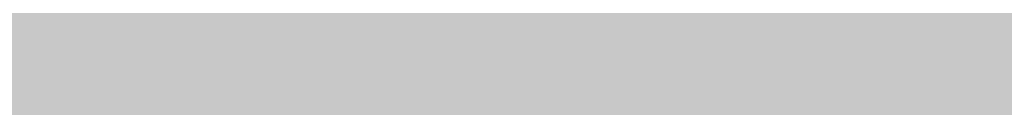
# Model space of a CAD drawing. Units: inches. Extents: x 2091 to 2899, y 967 to 2217.
# Tile 217 of 256: x 2203.2571 to 2203.4104, y 1152.2605 to 1152.274. Entities that reach past the tile are written whole.
import ezdxf

# ---------------------------------------------------------------- set-up
doc = ezdxf.new("R2010")
doc.units = ezdxf.units.IN
doc.layers.add('A-WALL-PATT', color=141, linetype='Continuous', lineweight=13, true_color=0xadddf7)

msp = doc.modelspace()

# ---------------------------------------------------------------- hatches: boundary and pattern name
at = {"layer": 'A-WALL-PATT'}
h = msp.add_hatch(color=256, dxfattribs=at)
h.dxf.hatch_style = 1
h.paths.add_polyline_path([(2803.1436, 2050.91906), (2203.1436, 2050.91906), (2203.1436, 1090.91906), (2803.1436, 1090.91906)])
h.paths.add_polyline_path([(2635.79885, 1147.54046), (2674.52405, 1147.54046, 0.376086), (2678.52967, 1152.8802), (2678.52967, 1159.55647, 0.333335), (2674.52432, 1163.56185), (2674.52432, 1163.56185), (2674.52432, 1192.93439), (2635.80597, 1192.93439), (2597.08762, 1192.93439), (2597.08762, 1163.56185, 0.333335), (2593.08228, 1159.55647), (2593.08228, 1152.8802, 0.376086), (2597.08789, 1147.54046)], flags=0)
h.paths.add_polyline_path([(2436.01043, 1278.24078, 0.000483), (2435.95264, 1278.21503, -0.001328), (2435.93563, 1278.11169, -0.001711), (2436.11644, 1278.04076, 0.002185)], flags=0)
h.paths.add_polyline_path([(2794.1436, 1143.41906), (2794.1436, 1347.41906), (2543.37017, 1347.41906), (2543.37017, 1351.91906), (2794.1436, 1351.91906), (2794.1436, 1392.71355), (2793.9474, 1392.71355), (2793.9474, 1473.5369), (2794.1436, 1473.5369), (2794.1436, 1531.91906), (2650.1436, 1531.91906), (2650.1436, 1536.41906), (2794.1436, 1536.41906), (2794.1436, 1692.41906), (2609.37561, 1692.41906), (2609.37561, 1644.41906), (2604.87561, 1644.41906), (2604.87561, 1744.91906), (2609.37561, 1744.91906), (2609.37561, 1696.91906), (2794.1436, 1696.91906), (2794.1436, 1780.91906), (2609.6436, 1780.91906), (2493.87561, 1780.91906), (2493.87561, 1785.41906), (2609.6436, 1785.41906), (2794.1436, 1785.41906), (2794.1436, 1847.93882), (2793.95122, 1847.93882), (2793.95122, 1928.76217), (2794.1436, 1928.76217), (2794.1436, 1941.41906), (2614.1436, 1941.41906), (2614.1436, 1821.41906), (2609.6436, 1821.41906), (2609.6436, 1941.41906), (2392.1436, 1941.41906), (2392.1436, 1819.91906), (2387.6436, 1819.91906), (2387.6436, 1941.41906), (2212.1436, 1941.41906), (2212.1436, 1783.91906), (2392.1436, 1783.91906), (2392.1436, 1780.91906), (2212.1436, 1780.91906), (2212.1436, 1629.41906), (2387.6436, 1629.41906), (2387.6436, 1744.91906), (2392.1436, 1744.91906), (2392.1436, 1627.91906), (2317.1436, 1627.91906), (2317.1436, 1551.41906), (2317.1436, 1536.41906), (2459.38359, 1536.41906), (2459.38359, 1602.39648), (2463.88359, 1602.39648), (2463.88359, 1531.91906), (2456.6436, 1531.91906), (2456.6436, 1529.91906), (2452.1436, 1529.91906), (2452.1436, 1531.91906), (2312.6436, 1531.91906), (2312.6436, 1551.41906), (2306.1436, 1551.41906), (2306.1436, 1555.91906), (2308.1436, 1555.91906), (2308.1436, 1551.41906), (2312.6436, 1551.41906), (2312.6436, 1627.91906), (2212.1436, 1627.91906), (2212.1436, 1555.91906), (2270.1436, 1555.91906), (2270.1436, 1551.41906), (2212.1436, 1551.41906), (2212.1436, 1351.91906), (2272.1436, 1351.91906), (2272.1436, 1347.41906), (2212.1436, 1347.41906), (2212.1436, 1275.41906), (2308.1436, 1275.41906), (2308.1436, 1351.91906), (2452.1436, 1351.91906), (2452.1436, 1493.91906), (2456.6436, 1493.91906), (2456.6436, 1347.41906), (2312.6436, 1347.41906), (2312.6436, 1270.91906), (2212.1436, 1270.91906), (2212.1436, 1099.91906), (2281.23752, 1099.91906), (2282.87104, 1110.9138), (2282.00834, 1116.9966), (2278.55774, 1121.4204), (2268.20564, 1128.0562), (2272.08764, 1128.0562), (2273.81294, 1131.927), (2279.42034, 1134.6919), (2285.02784, 1135.2449), (2287.61584, 1137.4568), (2288.04714, 1138.0098), (2289.34114, 1140.7747), (2291.06654, 1139.6687), (2292.36054, 1135.2449), (2295.37984, 1136.9038), (2296.24254, 1135.7979), (2297.10524, 1133.033), (2300.12464, 1138.0098), (2303.14394, 1138.0098), (2304.43794, 1135.7979), (2303.14394, 1133.586), (2306.59464, 1134.6919), (2307.88874, 1133.033), (2310.90804, 1135.2449), (2313.92744, 1134.1389), (2315.62686, 1132.4271), (2308.32004, 1117.5496), (2290.20384, 1109.8079), (2288.90984, 1103.1721), (2289.27231, 1099.91906), (2434.91823, 1099.91906), (2431.59323, 1124.78806), (2429.93023, 1169.55306), (2430.92718, 1240.51969), (2435.65893, 1238.18613), (2437.13523, 1196.55406), (2438.79823, 1143.97306), (2442.67823, 1111.99806), (2446.55823, 1099.91906), (2794.1436, 1099.91906), (2794.1436, 1138.91906), (2548.03245, 1138.91906), (2548.03245, 1143.41906), (2548.03245, 1148.81906), (2546.66846, 1148.03156), (2528.68569, 1179.17862, 0.256256), (2512.03245, 1148.81906), (2512.03245, 1143.41906), (2512.03245, 1138.91906), (2507.53245, 1138.91906), (2507.53245, 1143.41906), (2507.53245, 1148.81906, 0.256256), (2490.8792, 1179.17862), (2472.89644, 1148.03156), (2471.53245, 1148.81906), (2471.53245, 1143.41906), (2467.03245, 1143.41906), (2467.03245, 1269.94579, 0.039061), (2460.90999, 1273.58006), (2467.03245, 1273.58006), (2467.03245, 1286.32536, 0.014511), (2465.21619, 1286.76191), (2467.03245, 1287.05258), (2467.03245, 1323.41906), (2471.53245, 1323.41906), (2471.53245, 1148.81906), (2489.53245, 1179.99597), (2490.89644, 1179.20847), (2490.8792, 1179.17862, -0.256256), (2507.53245, 1148.81906), (2507.53245, 1143.41906), (2512.03245, 1143.41906), (2512.03245, 1148.81906, -0.256256), (2528.68569, 1179.17862), (2528.66846, 1179.20847), (2530.03245, 1179.99597), (2548.03245, 1148.81906), (2548.03245, 1143.41906)], flags=16)
h.paths.add_polyline_path([(2607.76855, 1200.94508), (2607.76855, 1265.03063), (2597.08762, 1281.05201), (2619.78459, 1281.05201), (2627.79528, 1337.12686), (2635.79885, 1337.12686), (2643.81666, 1337.12686), (2651.82736, 1281.05201), (2674.52432, 1281.05201), (2663.8434, 1265.03063), (2663.8434, 1200.94508), (2635.80597, 1200.94508)], flags=0)
edge = h.paths.add_edge_path(flags=0)
edge.add_ellipse((13303.89622, 1272.99872), major_axis=(-10595.31304, 0), ratio=0.84230387009, start_angle=0.628237219, end_angle=0.6465541, ccw=False)
edge.add_ellipse((2711.70045, 1156.85268), major_axis=(2.21977, 0), ratio=0.8423039, start_angle=111.53524, end_angle=180.62824, ccw=False)
edge.add_ellipse((13303.15629, 1272.99872), major_axis=(-10593.02631, 0), ratio=0.84230386954, start_angle=0.528271472, end_angle=0.646554097, ccw=False)
edge.add_line((2710.7646, 1175.3333), (2710.12999, 1175.3333))
edge.add_ellipse((2710.12999, 1176.57978), major_axis=(1.47985, 0), ratio=0.8423039, start_angle=180, end_angle=270, ccw=False)
edge.add_line((2708.65014, 1176.57978), (2708.65014, 1200.78291))
edge.add_ellipse((2710.12999, 1200.78291), major_axis=(1.47985, 0), ratio=0.8423039, start_angle=90, end_angle=180, ccw=False)
edge.add_line((2710.12999, 1202.02939), (2710.46508, 1202.02939))
edge.add_ellipse((13303.15629, 1272.99872), major_axis=(-10593.02631, 0), ratio=0.84230386954, start_angle=-0.090229089, end_angle=0.383866779, ccw=False)
edge.add_ellipse((2710.12999, 1290.92703), major_axis=(-1.47985, 0), ratio=0.8423039, start_angle=0, end_angle=90, ccw=False)
edge.add_line((2708.65014, 1290.92703), (2708.65014, 1315.13017))
edge.add_ellipse((2710.12999, 1315.13017), major_axis=(-1.47985, 0), ratio=0.8423039, start_angle=-90, end_angle=0, ccw=False)
edge.add_line((2710.12999, 1316.37665), (2710.70631, 1316.37665))
edge.add_ellipse((3238.40172, 1296.28957), major_axis=(528.234, 0), ratio=0.84230387, start_angle=176.3495724, end_angle=177.8200497, ccw=False)
edge.add_ellipse((2775.06304, 1071.4507), major_axis=(313.30776, 0), ratio=0.84230387, start_angle=102.1259656, end_angle=103.780529, ccw=False)
edge.add_ellipse((2775.06304, 1078.3057), major_axis=(-305.30289, 0), ratio=0.84230387, start_angle=-79.790461, end_angle=-77.5553727, ccw=False)
edge.add_ellipse((2695.14177, 1541.97538), major_axis=(-250.96022, 0), ratio=0.84230387, start_angle=99.256566, end_angle=102.5549326)
edge.add_line((2741.41033, 1334.21426), (2747.13255, 1337.37848))
edge.add_ellipse((2747.53862, 1336.85748), major_axis=(-0.73992, 0), ratio=0.842304, start_angle=270, end_angle=307.93313, ccw=False)
edge.add_ellipse((2747.53862, 1336.85748), major_axis=(-0.73992, 0), ratio=0.842304, start_angle=232.06687, end_angle=270, ccw=False)
edge.add_line((2747.94469, 1337.37848), (2753.66691, 1334.21426))
edge.add_ellipse((2799.93547, 1541.97538), major_axis=(250.96022, 0), ratio=0.84230387, start_angle=257.4450674, end_angle=260.743434)
edge.add_ellipse((2720.01419, 1078.3057), major_axis=(305.30289, 0), ratio=0.84230387, start_angle=77.5553727, end_angle=79.790461, ccw=False)
edge.add_ellipse((2720.01419, 1071.4507), major_axis=(-313.30776, 0), ratio=0.84230387, start_angle=256.219471, end_angle=257.8740344, ccw=False)
edge.add_ellipse((2256.67551, 1296.28957), major_axis=(-528.234, 0), ratio=0.84230387, start_angle=182.1799503, end_angle=183.6504276, ccw=False)
edge.add_line((2784.37092, 1316.37665), (2784.94725, 1316.37665))
edge.add_ellipse((2784.94725, 1315.13017), major_axis=(1.47985, 0), ratio=0.8423039, start_angle=0, end_angle=90, ccw=False)
edge.add_line((2786.42709, 1315.13017), (2786.42709, 1290.92703))
edge.add_ellipse((2784.94725, 1290.92703), major_axis=(1.47985, 0), ratio=0.8423039, start_angle=270, end_angle=360, ccw=False)
edge.add_ellipse((-7808.07906, 1272.99872), major_axis=(10593.02631, 0), ratio=0.84230386954, start_angle=-0.383866779, end_angle=0.090229089, ccw=False)
edge.add_line((2784.61216, 1202.02939), (2784.94725, 1202.02939))
edge.add_ellipse((2784.94725, 1200.78291), major_axis=(1.47985, 0), ratio=0.8423039, start_angle=0, end_angle=90, ccw=False)
edge.add_line((2786.42709, 1200.78291), (2786.42709, 1176.57978))
edge.add_ellipse((2784.94725, 1176.57978), major_axis=(-1.47985, 0), ratio=0.8423039, start_angle=90, end_angle=180, ccw=False)
edge.add_line((2784.94725, 1175.3333), (2784.31264, 1175.3333))
edge.add_ellipse((-7808.07906, 1272.99872), major_axis=(10593.02631, 0), ratio=0.84230386954, start_angle=-0.618643196, end_angle=-0.528271472, ccw=False)
edge.add_ellipse((2783.37678, 1156.85268), major_axis=(-2.21977, 0), ratio=0.8423039, start_angle=179.37176, end_angle=248.46476, ccw=False)
edge.add_ellipse((-7808.81898, 1272.99872), major_axis=(-10595.31304, 0), ratio=0.84230386576, start_angle=179.353445923, end_angle=179.371762803, ccw=False)
edge.add_ellipse((2780.2973, 1153.50079), major_axis=(-5.24643, 0), ratio=0.8423039, start_angle=90, end_angle=179.35345, ccw=False)
edge.add_line((2780.2973, 1149.08171), (2714.77993, 1149.08171))
edge.add_ellipse((2714.77993, 1153.50079), major_axis=(5.24643, 0), ratio=0.8423039, start_angle=180.64655, end_angle=270, ccw=False)
edge = h.paths.add_edge_path(flags=0)
edge.add_line((2718.18737, 1151.00783), (2718.18737, 1170.47236))
edge.add_ellipse((2721.14706, 1170.47236), major_axis=(-2.95969, 0), ratio=0.8423039, start_angle=-90, end_angle=0, ccw=False)
edge.add_line((2721.14706, 1172.96532), (2773.93017, 1172.96532))
edge.add_ellipse((2773.93017, 1170.47236), major_axis=(-2.95969, 0), ratio=0.8423039, start_angle=180, end_angle=270, ccw=False)
edge.add_line((2776.88987, 1170.47236), (2776.88987, 1151.00783))
edge.add_line((2776.88987, 1151.00783), (2718.18737, 1151.00783))
edge = h.paths.add_edge_path(flags=0)
edge.add_line((2718.18737, 1180.23415), (2718.18737, 1199.05783))
edge.add_ellipse((2747.53862, 1320.39864), major_axis=(147.01792, 0), ratio=0.84230387, start_angle=256.4018653, end_angle=283.5981347)
edge.add_line((2776.88987, 1199.05783), (2776.88987, 1180.23415))
edge.add_ellipse((2747.53862, 1301.57496), major_axis=(147.01792, 0), ratio=0.84230387, start_angle=256.4018653, end_angle=283.5981347, ccw=False)
edge = h.paths.add_edge_path(flags=0)
edge.add_ellipse((13303.15629, 1272.99872), major_axis=(-10591.54646, 0), ratio=0.84230386955, start_angle=0.055594314, end_angle=0.377764194, ccw=False)
edge.add_line((2711.61686, 1262.72171), (2715.66741, 1249.4954))
edge.add_ellipse((6413.89196, 1241.69192), major_axis=(-3698.23616, 0), ratio=0.8423038695, start_angle=-0.12089737, end_angle=0.36407635)
edge.add_line((2715.76104, 1218.19245), (2711.93431, 1203.16736))
edge = h.paths.add_edge_path(flags=0)
edge.add_line((2718.18737, 1251.07457), (2716.00249, 1267.45044))
edge.add_ellipse((2742.15117, 1202.18954), major_axis=(81.77258, 0), ratio=0.84230387, start_angle=94.277421, end_angle=111.8349538, ccw=False)
edge.add_line((2737.00975, 1270.93063), (2758.06748, 1270.93063))
edge.add_ellipse((2752.92606, 1202.18954), major_axis=(81.77258, 0), ratio=0.84230387, start_angle=68.1650462, end_angle=85.722579, ccw=False)
edge.add_line((2779.07475, 1267.45044), (2776.88987, 1251.07457))
edge.add_ellipse((2750.33806, 1187.88536), major_axis=(79.57966, 0), ratio=0.84230387, start_angle=67.2080851, end_angle=85.1299304)
edge.add_line((2756.03466, 1254.74366), (2739.04258, 1254.74366))
edge.add_ellipse((2744.73917, 1187.88536), major_axis=(79.57966, 0), ratio=0.84230387, start_angle=94.8700696, end_angle=112.7919149)
edge = h.paths.add_edge_path(flags=0)
edge.add_line((2783.14293, 1203.16736), (2779.31619, 1218.19245))
edge.add_ellipse((-918.81473, 1241.69192), major_axis=(3698.23616, 0), ratio=0.8423038695, start_angle=-0.36407635, end_angle=0.12089737)
edge.add_line((2779.40983, 1249.4954), (2783.46037, 1262.72171))
edge.add_ellipse((-7808.07906, 1272.99872), major_axis=(-10591.54646, 0), ratio=0.84230386954, start_angle=179.622235806, end_angle=179.944405687, ccw=False)
edge = h.paths.add_edge_path(flags=0)
edge.add_ellipse((2734.20089, 1286.69044), major_axis=(-0.35661, 6.34008), ratio=0.6038336, start_angle=89.002014, end_angle=253.657408, ccw=False)
edge.add_line((2730.369, 1286.54181), (2730.369, 1301.35198))
edge.add_line((2730.369, 1301.35198), (2735.91331, 1305.2148))
edge.add_ellipse((2736.38492, 1304.73456), major_axis=(0.73992, 0), ratio=0.842304, start_angle=90, end_angle=134.48021, ccw=False)
edge.add_line((2736.38492, 1305.3578), (2738.03278, 1305.3578))
edge.add_line((2738.03278, 1305.3578), (2738.03278, 1307.70793))
edge.add_ellipse((2794.20164, 1307.70793), major_axis=(56.16886, 0), ratio=0.84230387, start_angle=150.56143, end_angle=180, ccw=False)
edge.add_ellipse((2700.87559, 1307.70793), major_axis=(-56.16886, 0), ratio=0.84230387, start_angle=180, end_angle=209.43857, ccw=False)
edge.add_line((2757.04445, 1307.70793), (2757.04445, 1305.3578))
edge.add_line((2757.04445, 1305.3578), (2758.69232, 1305.3578))
edge.add_ellipse((2758.69232, 1304.73456), major_axis=(-0.73992, 0), ratio=0.842304, start_angle=225.51979, end_angle=270, ccw=False)
edge.add_line((2759.16392, 1305.2148), (2764.70823, 1301.35198))
edge.add_line((2764.70823, 1301.35198), (2764.70823, 1286.54181))
edge.add_ellipse((2760.87634, 1286.69044), major_axis=(0.35661, 6.34008), ratio=0.6038336, start_angle=106.342592, end_angle=270.997986, ccw=False)
edge.add_line((2757.04445, 1285.79709), (2757.04445, 1307.70793))
edge.add_ellipse((2700.87559, 1307.70793), major_axis=(-56.16886, 0), ratio=0.84230387, start_angle=180, end_angle=209.43857)
edge.add_ellipse((2794.20164, 1307.70793), major_axis=(56.16886, 0), ratio=0.84230387, start_angle=150.56143, end_angle=180)
edge.add_line((2738.03278, 1307.70793), (2738.03278, 1285.79709))
h.paths.add_polyline_path([(2417.81227, 1104.4497), (2413.49227, 1102.5297), (2410.61227, 1103.9697), (2409.17227, 1106.3697), (2407.25227, 1107.3297), (2406.29227, 1109.7297), (2405.33227, 1114.0497), (2405.33227, 1117.8897), (2406.29227, 1120.1297), (2407.25227, 1119.8097), (2408.84832, 1118.32766), (2410.17395, 1119.42417), (2410.21127, 1120.4057), (2411.04073, 1121.41905), (2410.69927, 1119.8587), (2410.17395, 1119.42417), (2410.08845, 1117.17611), (2411.13284, 1116.20632), (2413.97227, 1119.3297), (2416.85227, 1120.7697), (2416.86972, 1120.79878), (2417.03507, 1119.40512), (2417.89621, 1118.14338), (2418.29227, 1118.3697), (2419.54445, 1120.03927), (2419.36092, 1118.38749), (2419.03211, 1119.35615), (2418.39894, 1118.51193), (2419.25227, 1114.5297), (2418.79409, 1107.19879)], flags=0)
h.paths.add_polyline_path([(2508.87017, 1347.41906), (2508.37017, 1347.41906), (2508.37017, 1351.91906), (2508.87017, 1351.91906)], flags=0)
h.paths.add_polyline_path([(2473.37017, 1347.41906), (2472.37017, 1347.41906), (2467.87017, 1347.41906), (2467.87017, 1455.41906), (2472.37017, 1455.41906), (2472.37017, 1352.41906), (2473.37017, 1352.41906)], flags=0)
h.paths.add_polyline_path([(2352.10624, 1217.4462), (2349.22624, 1218.8862), (2347.78624, 1221.2862), (2345.86624, 1222.2462), (2344.90624, 1224.6462), (2343.94624, 1228.9662), (2343.94624, 1232.8062), (2344.90624, 1235.0462), (2345.86624, 1234.7262), (2347.46229, 1233.24415), (2348.78792, 1234.34066), (2348.82524, 1235.3222), (2349.6547, 1236.33555), (2349.31324, 1234.7752), (2348.78792, 1234.34066), (2348.70242, 1232.0926), (2349.74681, 1231.12282), (2352.58624, 1234.2462), (2355.46624, 1235.6862), (2355.48369, 1235.71528), (2355.64904, 1234.32161), (2356.51018, 1233.05988), (2356.90624, 1233.2862), (2358.15842, 1234.95576), (2357.97489, 1233.30398), (2357.64608, 1234.27264), (2357.01291, 1233.42842), (2357.86624, 1229.4462), (2357.40806, 1222.11529), (2356.42624, 1219.3662)], flags=0)
h.paths.add_polyline_path([(2348.2968, 1112.22442), (2347.0138, 1112.31042), (2345.5298, 1114.12742), (2345.7318, 1115.85842), (2346.8118, 1116.98242), (2346.8118, 1114.64642), (2345.8668, 1114.21442), (2346.8798, 1114.30042)], flags=0)
h.paths.add_polyline_path([(2347.0138, 1110.92642), (2346.2718, 1110.49342), (2346.6098, 1111.18642)], flags=0)
h.paths.add_polyline_path([(2345.8668, 1118.19442), (2345.5298, 1117.32942), (2343.7078, 1118.02142), (2344.3828, 1118.62642)], flags=0)
h.paths.add_polyline_path([(2346.6768, 1109.28242), (2346.0698, 1108.07142), (2345.8668, 1110.06142)], flags=0)
h.paths.add_polyline_path([(2345.0568, 1119.75142), (2343.6398, 1119.75142), (2343.9778, 1121.13542)], flags=0)
h.paths.add_polyline_path([(2345.2598, 1116.55042), (2345.1248, 1115.85842), (2344.9218, 1115.68542), (2344.7198, 1116.37742)], flags=0)
h.paths.add_polyline_path([(2345.6648, 1112.31042), (2345.4618, 1111.53242), (2344.0448, 1111.96442), (2344.6518, 1112.57042)], flags=0)
h.paths.add_polyline_path([(2345.1918, 1113.34942), (2344.4498, 1113.86842), (2344.7198, 1114.38742)], flags=0)
h.paths.add_polyline_path([(2344.6518, 1116.80942), (2344.1798, 1115.68542), (2344.6518, 1115.33942), (2343.9098, 1114.90642), (2343.0328, 1115.94442), (2343.6398, 1116.46342)], flags=0)
h.paths.add_polyline_path([(2345.8668, 1106.68642), (2344.9898, 1105.56242), (2344.5168, 1106.60042)], flags=0)
h.paths.add_polyline_path([(2344.8548, 1110.06142), (2344.5168, 1109.28242), (2344.1128, 1109.71542)], flags=0)
h.paths.add_polyline_path([(2344.0448, 1113.52242), (2343.4378, 1113.08942), (2342.7628, 1113.95442)], flags=0)
h.paths.add_polyline_path([(2344.3148, 1111.01242), (2342.9648, 1110.32042), (2342.9648, 1111.09942)], flags=0)
h.paths.add_polyline_path([(2345.1248, 1104.69742), (2344.5848, 1103.74542), (2344.4498, 1104.26442)], flags=0)
h.paths.add_polyline_path([(2342.8298, 1121.22242), (2341.7498, 1120.53042), (2340.5358, 1121.04942), (2340.1308, 1121.82842), (2340.6708, 1122.95242), (2341.1428, 1121.82842), (2341.6148, 1122.00142)], flags=0)
h.paths.add_polyline_path([(2342.9648, 1119.75142), (2343.0328, 1118.45342), (2342.0878, 1118.02142), (2342.0198, 1119.49142)], flags=0)
h.paths.add_polyline_path([(2342.6948, 1116.89642), (2341.9528, 1116.63642), (2342.0198, 1117.32942)], flags=0)
h.paths.add_polyline_path([(2343.0328, 1112.22442), (2342.0198, 1111.79142), (2341.5478, 1112.22442), (2342.3578, 1113.34942)], flags=0)
h.paths.add_polyline_path([(2343.7748, 1104.43742), (2342.6278, 1102.88042), (2342.6948, 1104.61042), (2343.4378, 1105.12942)], flags=0)
h.paths.add_polyline_path([(2342.0198, 1115.07942), (2340.8058, 1115.51242), (2340.9408, 1116.37742)], flags=0)
h.paths.add_polyline_path([(2341.4808, 1120.09742), (2341.4808, 1119.40542), (2341.0758, 1119.57842), (2341.1428, 1120.09742)], flags=0)
h.paths.add_polyline_path([(2341.8178, 1114.47342), (2340.9408, 1113.08942), (2340.8058, 1114.56042)], flags=0)
h.paths.add_polyline_path([(2341.1428, 1118.54042), (2340.9408, 1116.98242), (2339.0508, 1117.67542), (2339.0508, 1118.62642)], flags=0)
h.paths.add_polyline_path([(2342.6948, 1101.66842), (2341.9528, 1101.84142), (2342.5598, 1102.36142)], flags=0)
h.paths.add_polyline_path([(2340.3328, 1119.66542), (2338.4438, 1119.57842), (2337.9038, 1120.35742), (2339.6578, 1120.61642)], flags=0)
h.paths.add_polyline_path([(2340.3328, 1115.33942), (2340.0628, 1113.69542), (2339.3878, 1115.33942)], flags=0)
h.paths.add_polyline_path([(2341.8178, 1103.83142), (2341.5478, 1102.88042), (2341.1428, 1103.65842)], flags=0)
h.paths.add_polyline_path([(2339.0508, 1122.86642), (2337.2958, 1121.82842), (2337.0938, 1123.12542), (2337.7688, 1123.81842)], flags=0)
h.paths.add_polyline_path([(2339.1178, 1121.74142), (2338.8478, 1121.22242), (2338.1738, 1121.04942), (2338.3758, 1121.56842)], flags=0)
h.paths.add_polyline_path([(2339.1858, 1119.31942), (2338.6458, 1118.71342), (2338.2408, 1118.10742), (2338.2408, 1118.88642)], flags=0)
h.paths.add_polyline_path([(2341.1428, 1101.92842), (2340.6028, 1101.23642), (2340.0628, 1101.84142), (2340.6028, 1102.36142)], flags=0)
h.paths.add_polyline_path([(2337.6338, 1117.76142), (2336.6208, 1118.28042), (2337.2958, 1118.97242)], flags=0)
h.paths.add_polyline_path([(2336.8238, 1119.57842), (2334.7988, 1118.97242), (2335.2038, 1120.35742), (2336.5538, 1120.87642)], flags=0)
h.paths.add_polyline_path([(2339.1178, 1100.45742), (2337.3638, 1100.54342), (2336.7558, 1101.23642)], flags=0)
h.paths.add_polyline_path([(2336.3508, 1122.43342), (2336.0138, 1121.91442), (2334.9338, 1122.43342), (2334.5288, 1123.47142), (2335.7438, 1122.77942)], flags=0)
h.paths.add_polyline_path([(2334.7318, 1120.87642), (2334.2588, 1120.35742), (2334.0568, 1120.78942), (2334.5968, 1121.30842)], flags=0)
h.paths.add_polyline_path([(2334.4618, 1122.17442), (2332.5718, 1121.30842), (2331.3568, 1122.17442), (2332.0998, 1122.86642)], flags=0)
h.paths.add_polyline_path([(2334.2588, 1118.54042), (2333.3818, 1118.45342), (2333.6518, 1119.31942)], flags=0)
h.paths.add_polyline_path([(2335.5418, 1102.27442), (2334.1918, 1102.62042), (2335.2718, 1103.31242)], flags=0)
h.paths.add_polyline_path([(2332.7068, 1119.66542), (2331.6948, 1120.44342), (2332.5048, 1120.78942)], flags=0)
h.paths.add_polyline_path([(2334.7318, 1101.14942), (2333.5168, 1101.58242), (2333.9888, 1101.75542)], flags=0)
h.paths.add_polyline_path([(2332.6398, 1116.63642), (2331.0868, 1116.29042), (2331.9648, 1118.19442)], flags=0)
h.paths.add_polyline_path([(2330.7498, 1121.56842), (2330.2768, 1120.27042), (2328.5228, 1119.31942), (2328.9948, 1121.04942)], flags=0)
h.paths.add_polyline_path([(2330.7498, 1118.62642), (2330.0078, 1117.50242), (2329.8728, 1118.02142)], flags=0)
h.paths.add_polyline_path([(2332.0998, 1102.36142), (2330.5468, 1102.01442), (2331.6948, 1102.96642)], flags=0)
h.paths.add_polyline_path([(2329.5348, 1113.60842), (2329.0628, 1112.31042), (2328.5898, 1113.34942)], flags=0)
h.paths.add_polyline_path([(2328.3878, 1117.84842), (2327.5098, 1116.55042), (2327.1728, 1117.76142)], flags=0)
h.paths.add_polyline_path([(2329.7378, 1106.51342), (2329.5348, 1105.30242), (2328.2528, 1106.08142)], flags=0)
h.paths.add_polyline_path([(2328.6578, 1114.38742), (2328.0498, 1114.12742), (2328.3198, 1114.90642)], flags=0)
h.paths.add_polyline_path([(2328.3198, 1112.22442), (2327.1058, 1112.13742), (2326.7008, 1112.65642)], flags=0)
h.paths.add_polyline_path([(2326.9028, 1115.25242), (2326.7008, 1114.12742), (2325.2158, 1113.60842), (2326.0928, 1115.33942)], flags=0)
h.paths.add_polyline_path([(2326.6328, 1108.33042), (2326.0928, 1107.37942), (2325.8908, 1108.50342), (2326.4978, 1109.10942)], flags=0)
h.paths.add_polyline_path([(2615.1436, 1531.91906), (2609.6436, 1531.91906), (2609.6436, 1620.41906), (2614.1436, 1620.41906), (2614.1436, 1536.41906), (2615.1436, 1536.41906)], flags=0)
h.paths.add_polyline_path([(2545.1436, 1563.41906), (2464.1436, 1563.41906), (2464.1436, 1632.41906), (2509.1436, 1632.41906), (2509.1436, 1627.91906), (2509.1436, 1603.91906), (2468.6436, 1603.91906), (2468.6436, 1567.91906), (2540.6436, 1567.91906), (2540.6436, 1591.91906), (2545.1436, 1591.91906)], flags=0)
h.paths.add_polyline_path([(2388.96905, 1549.98573), (2357.43418, 1549.98573), (2357.43418, 1623.36078), (2399.36278, 1623.36078), (2435.68947, 1623.36078), (2435.59255, 1602.55927), (2435.59255, 1602.39648), (2388.96905, 1602.39648)], flags=0)
h.paths.add_polyline_path([(2388.88063, 1555.80915), (2374.90443, 1555.80915), (2374.90443, 1600.57156), (2374.90443, 1615.45765), (2406.35088, 1615.45765), (2406.35088, 1618.93943), (2412.17429, 1615.45765), (2406.35088, 1611.97586), (2406.35088, 1615.45765), (2388.88063, 1615.45765)], flags=0)
h.paths.add_polyline_path([(2568.87561, 1644.41906), (2453.37561, 1644.41906), (2453.37561, 1785.41906), (2457.87561, 1785.41906), (2457.87561, 1648.91906), (2568.87561, 1648.91906)], flags=0)
h.paths.add_polyline_path([(2212.1436, 1945.91906), (2212.1436, 2041.91906), (2794.1436, 2041.91906), (2794.1436, 1945.91906)], flags=16)
h.paths.add_polyline_path([(2271.08273, 1964.31724), (2776.85297, 1964.31724), (2776.85297, 2037.16962), (2271.08273, 2037.16962)], flags=8)
h.paths.add_polyline_path([(2380.64929, 1536.82414), (2461.04081, 1536.82414), (2461.04081, 1554.65259), (2380.64929, 1554.65259)], flags=8)
h.paths.add_polyline_path([(2240.75571, 1609.72545), (2309.18583, 1609.72545), (2309.18583, 1617.6982), (2240.75571, 1617.6982)], flags=8)
h.paths.add_polyline_path([(2212.67726, 1313.5041), (2282.59152, 1313.5041), (2282.59152, 1322.74524), (2212.67726, 1322.74524)], flags=8)
h.paths.add_polyline_path([(2457.11198, 1114.77857), (2558.48158, 1114.77857), (2558.48158, 1142.21968), (2457.11198, 1142.21968)], flags=8)
h.paths.add_polyline_path([(2473.44234, 1273.01007), (2604.64123, 1273.01007), (2604.64123, 1318.34693), (2473.44234, 1318.34693)], flags=8)
h.paths.add_polyline_path([(2638.8763, 1626.97743), (2684.25037, 1627.97674), (2684.03848, 1637.59749), (2638.66442, 1636.59819)], flags=8)
h.paths.add_polyline_path([(2537.59055, 1453.79345), (2628.38955, 1453.79345), (2628.38955, 1475.34481), (2537.59055, 1475.34481)], flags=8)
h.paths.add_polyline_path([(2504.13764, 1714.6324), (2554.64719, 1714.6324), (2554.64719, 1730.23771), (2504.13764, 1730.23771)], flags=8)
h.paths.add_polyline_path([(2487.50118, 1575.65187), (2535.09712, 1575.65187), (2535.09712, 1598.37765), (2487.50118, 1598.37765)], flags=8)
h.paths.add_polyline_path([(2709.0994, 1735.71028), (2740.0166, 1735.71028), (2740.0166, 1749.93764), (2709.0994, 1749.93764)], flags=8)
h.paths.add_polyline_path([(2442.43842, 1792.17166), (2564.72884, 1792.17166), (2564.72884, 1842.00016), (2442.43842, 1842.00016)], flags=8)
h.paths.add_polyline_path([(2655.8158, 1809.64408), (2789.52014, 1806.6938), (2790.08498, 1832.29164), (2656.38064, 1835.24192)], flags=8)
h.paths.add_polyline_path([(2234.8427, 1797.72014), (2368.59285, 1794.76885), (2369.16072, 1820.50413), (2235.41056, 1823.45542)], flags=8)
h.paths.add_polyline_path([(2245.13847, 1644.00633), (2398.42773, 1640.6239), (2398.99484, 1666.32482), (2245.70557, 1669.70725)], flags=8)
h.paths.add_polyline_path([(2306.14285, 1431.16852), (2413.76831, 1428.79369), (2414.33315, 1454.39153), (2306.70768, 1456.76636)], flags=8)
h.paths.add_polyline_path([(2306.83458, 1458.23314), (2393.38048, 1456.32345), (2393.93281, 1481.35436), (2307.38691, 1483.26405)], flags=8)

doc.saveas('drawing.dxf')
